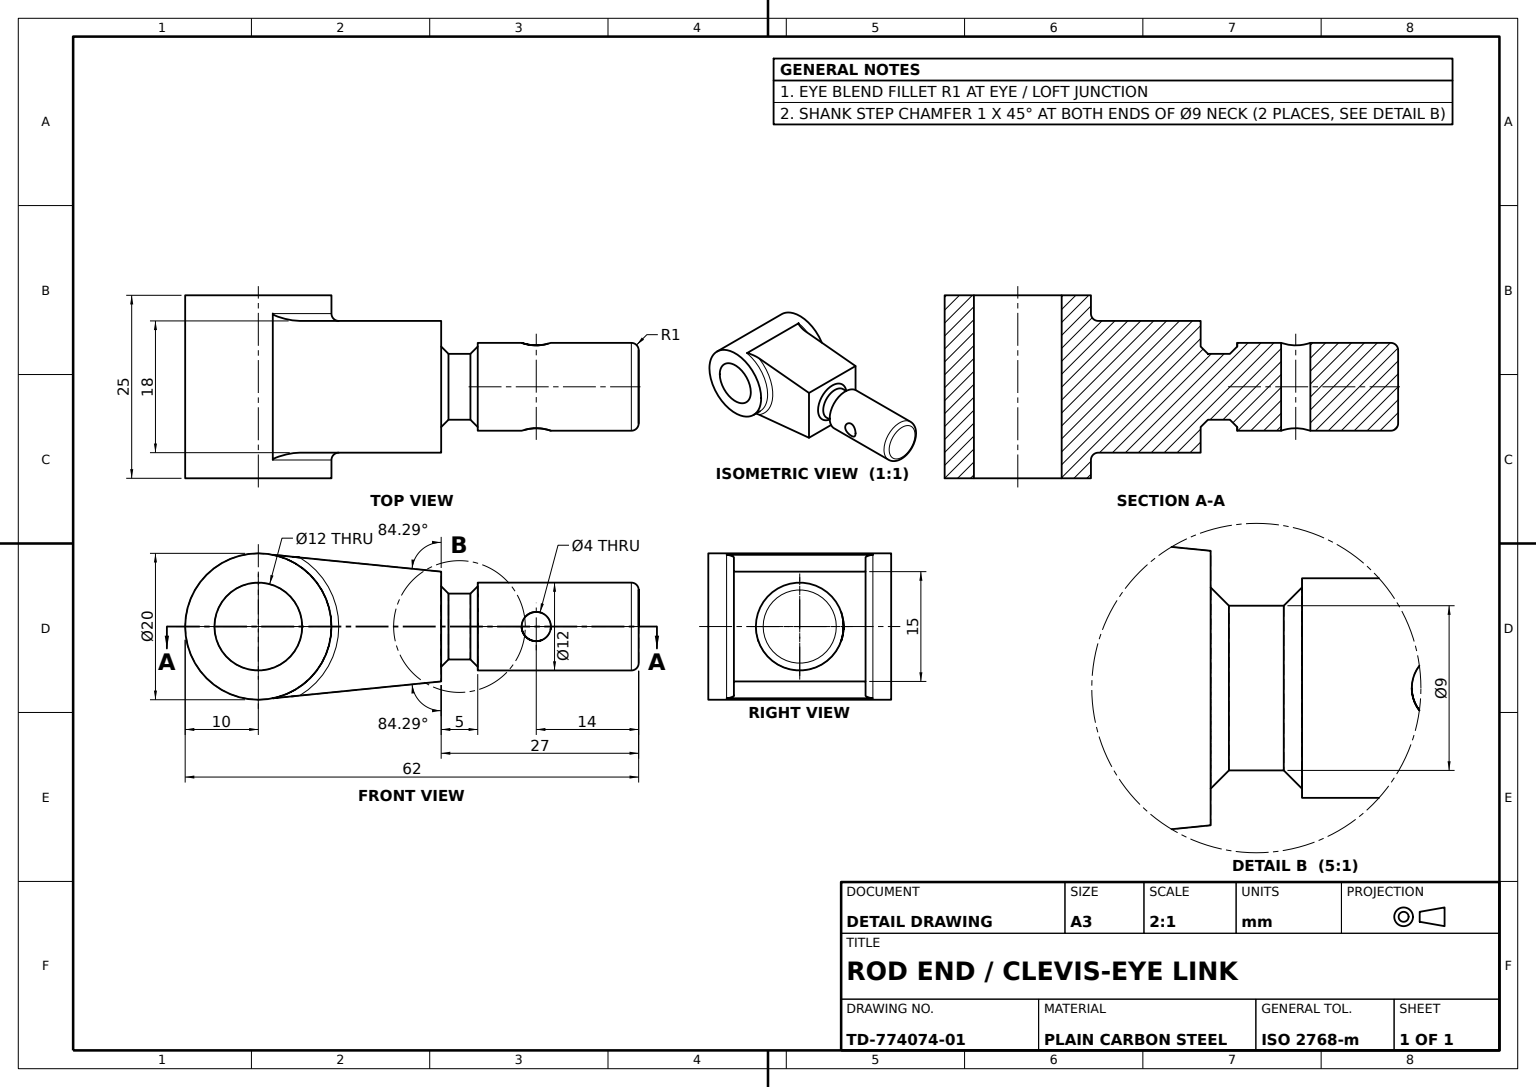
from build123d import *

# Parameters (mm, degrees)
SHANK_PROFILE_12_R           = 6
SHANK_12X27_DEPTH            = 27
SHANK_STEP_9X5_DEPTH         = 29.301943396
SHANK_STEP_9X5_DEPTH_BACK    = 5
SHANK_STEP_PROFILE_9_R       = 6
SHANK_STEP_PROFILE_9_R_2     = 4.5
EYE_PROFILE_20_R             = 10
EYE_PROFILE_20_R_2           = 6
EYE_BOSS_20X25_DEPTH         = 12.5
EYE_START                    = -35
EYE_BORE_PROFILE_R           = 6
EYE_BORE_DEPTH               = 35
CROSS_HOLE_4_DEPTH           = 65.033194649
CROSS_HOLE_4_DEPTH_BACK      = 65.033194649
CROSS_HOLE_PROFILE_4_R       = 2
EYE_BLEND_FILLET_R1_R        = 1
SHANK_STEP_CHAMFER_1X45_SIZE = 1


with BuildPart() as part:
    # Shank Profile Ø12 → Shank Ø12x27 (new body)
    with BuildSketch(Plane.XY):
        Circle(SHANK_PROFILE_12_R)
    extrude(amount=SHANK_12X27_DEPTH)

    # Shank Step Profile Ø9 → Shank Step Ø9x5 (cut, two sides: drawn at the far end of the back side and taken through both)
    with BuildSketch(Plane.XY.offset(27).offset(-SHANK_STEP_9X5_DEPTH_BACK)):
        Circle(SHANK_STEP_PROFILE_9_R)
        Circle(SHANK_STEP_PROFILE_9_R_2, mode=Mode.SUBTRACT)
    extrude(amount=SHANK_STEP_9X5_DEPTH + SHANK_STEP_9X5_DEPTH_BACK, mode=Mode.SUBTRACT)



with BuildPart() as body_2:
    # Eye Profile Ø20 → Eye Boss Ø20x25 (new, symmetric)
    with BuildSketch(Plane(origin=(0, 0, 0), x_dir=(0, 0, -1), z_dir=(1, 0, 0))):
        with Locations((-52, 0)):
            Circle(EYE_PROFILE_20_R)
        with Locations((-52, 0)):
            Circle(EYE_PROFILE_20_R_2, mode=Mode.SUBTRACT)
    extrude(amount=EYE_BOSS_20X25_DEPTH, both=True)


with BuildPart() as part_1:
    add(part.part)

    add(body_2.part)  # Shank To Eye Transition merges body 2
    # Loft End Section 18x20 → Shank To Eye Transition section 0
    with BuildSketch(Plane.XY.offset(52)):
        with BuildLine():
            Line((-9, 10), (9, 10))
            Line((9, 10), (9, -10))
            Line((9, -10), (-9, -10))
            Line((-9, -10), (-9, 10))
        make_face()
    # Loft Start Section 18x15 → Shank To Eye Transition section 1
    with BuildSketch(Plane.XY.offset(27)):
        with BuildLine():
            Line((-9, 7.5), (9, 7.5))
            Line((9, 7.5), (9, -7.5))
            Line((9, -7.5), (-9, -7.5))
            Line((-9, -7.5), (-9, 7.5))
        make_face()
    loft()

    # Eye Bore Profile → Eye Bore (cut)
    with BuildSketch(Plane(origin=(12.5, 0, 0), x_dir=(0, 0, -1), z_dir=(1, 0, 0)).offset(EYE_START)):
        with Locations((-52, 0)):
            Circle(EYE_BORE_PROFILE_R)
    extrude(amount=EYE_BORE_DEPTH, mode=Mode.SUBTRACT)

    # Cross Hole Profile Ø4 → Cross Hole Ø4 (cut, two sides: drawn at the far end of the back side and taken through both)
    with BuildSketch(Plane(origin=(0, 0, 0), x_dir=(0, 0, -1), z_dir=(1, 0, 0)).offset(-CROSS_HOLE_4_DEPTH_BACK)):
        with Locations(Location((-14, 0, 0), (0, 0, 180))):
            Circle(CROSS_HOLE_PROFILE_4_R)
    extrude(amount=CROSS_HOLE_4_DEPTH + CROSS_HOLE_4_DEPTH_BACK, mode=Mode.SUBTRACT)

    # Eye Blend Fillet R1
    eye_blend_fillet_r1_edges = [part_1.edges().sort_by_distance(p)[0] for p in [
        (-9, -6.332377898, 44.260427013),
        (9, 6.332377898, 44.260427013),
        (-6, 0, 0),
    ]]
    fillet(eye_blend_fillet_r1_edges, radius=EYE_BLEND_FILLET_R1_R)

    # Shank Step Chamfer 1x45
    shank_step_chamfer_1x45_edges = [part_1.edges().sort_by_distance(p)[0] for p in [
        (-4.5, 0, 27),
        (-4.5, 0, 22),
    ]]
    chamfer(shank_step_chamfer_1x45_edges, length=SHANK_STEP_CHAMFER_1X45_SIZE)


solid = part_1.part
